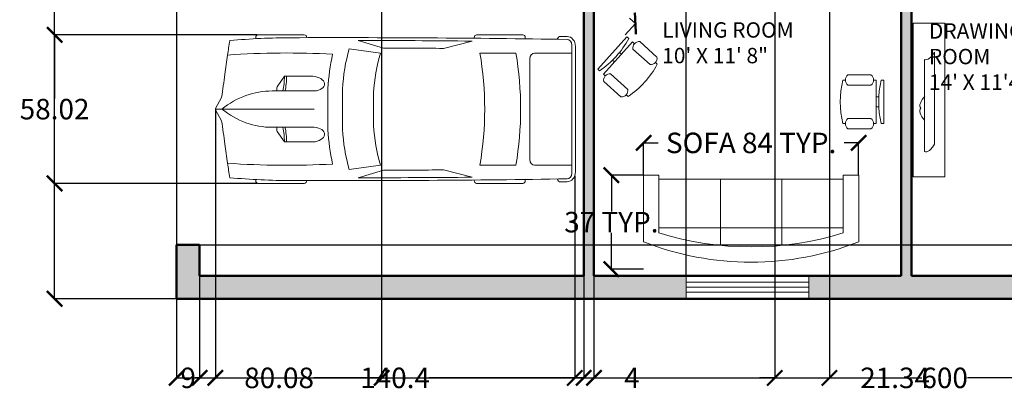
# Model space of a CAD drawing. Units: inches. Extents: x -30 to 744, y -375 to 57.
# Tile 1 of 8: x -30 to 355, y -375 to -230. Entities that reach past the tile are written whole.
import ezdxf

# ---------------------------------------------------------------- set-up
doc = ezdxf.new("R2010")
doc.units = ezdxf.units.IN
doc.header["$MEASUREMENT"] = 0
for name, color, linetype, lineweight in [('A-ANNO-DIMS', 2, 'Continuous', 18), ('A-AREA-IDEN', 7, 'Continuous', 25), ('A-EQPM-VEHI', 8, 'Continuous', 13), ('A-FURN', 8, 'Continuous', 18), ('A-GLAZ', 4, 'Continuous', 18), ('A-WALL', 7, 'Continuous', 50)]:
    doc.layers.add(name, color=color, linetype=linetype, lineweight=lineweight)
doc.layers.add('A-WALL-PATT', color=251, linetype='Continuous', lineweight=13, true_color=0x636466)
doc.styles.get("Standard").update_dxf_attribs({"font": 'arial.ttf'})
doc.dimstyles.get("Standard").update_dxf_attribs({"dimtxt": 8, "dimasz": 6, "dimexe": 0.18, "dimexo": 0.0625, "dimgap": 0.09, "dimtad": 0, "dimtih": 1, "dimtoh": 1, "dimdec": 0, "dimzin": 0, "dimdsep": 46, "dimlunit": 4, "dimtxsty": 'Standard', "dimblk": 'ARCHTICK', "dimcen": 0.09, "dimadec": 0, "dimazin": 0, "dimtfac": 1, "dimtdec": 0, "dimtofl": 0, "dimtmove": 0, "dimatfit": 1, "dimldrblk": 'ARCHTICK', "dimfxl": 1, "dimtolj": 1, "dimtzin": 0, "dimarcsym": 0})

# ---------------------------------------------------------------- blocks, each defined once
blk = doc.blocks.new('Sofa - Roundback 7 ft.')
for p, q in [((-12.00002, -32.4421), (-12.00003, -6.5971)), ((11.99997, -32.4421), (11.99998, -6.5971)), ((-36.000027, -34), (-36.000027, -11.4696)), ((35.99998, -34), (35.99998, -11.4696)), ((-35.999844, -13.3819), (35.9998, -13.3819)), ((-36.000027, -32.4421), (35.99998, -32.4421))]:
    blk.add_line(p, q)
for points in [[(-36.000027, -34), (-42.000027, -34), (-42.000027, -8)], [(41.99998, -8), (41.99998, -34), (35.99998, -34)]]:
    blk.add_lwpolyline(points)
for centre, radius, start, end in [((0, -114.25), 114.25, 68.43141, 111.5686), ((-0.00001, -127.1968), 121.1968, 72.72033, 107.2797)]:
    blk.add_arc(centre, radius, start, end)
blk = doc.blocks.new('Chair - Desk')
for p, q in [((-8.5, 0), (-8.5, -1)), ((-8.5, 0), (8.5, 0)), ((8.5, 0), (8.5, -1)), ((-8.5, -3), (-8.5, -4)), ((-8.5, -3), (8.5, -3)), ((-2, -3), (-2, -1.9355)), ((2, -1.9576), (2, -3)), ((8.5, -3), (8.5, -4)), ((-10.5, -5), (-10.5, -14)), ((-6.5, -14), (-6.5, -5)), ((6.5, -5), (6.5, -14)), ((10.5, -14), (10.5, -5)), ((-8.5, -15), (-8.5, -16)), ((8.5, -15), (8.5, -16))]:
    blk.add_line(p, q)
for centre, radius, start, end in [((0, 34.625), 36.625, 256.5803, 283.4197), ((-8.5, -6.5), 2.5, 36.8699, 143.1301), ((8.5, -6.5), 2.5, 36.8699, 143.1301), ((-8.5, -12.5), 2.5, 216.8699, 323.1301), ((8.5, -12.5), 2.5, 216.8699, 323.1301), ((0, 19.625), 36.625, 256.5803, 283.4197)]:
    blk.add_arc(centre, radius, start, end)
blk = doc.blocks.new('*U20')
for p, q in [((21.1, 37.41), (21.1, 36.83)), ((46.55, 38.89), (22.35, 38.89)), ((47.8, 37.39), (47.8, 37.41)), ((135.45, 37.07), (135.45, 37.41)), ((136.7, 38.89), (160.9, 38.89)), ((162.15, 37.41), (162.15, 36.77)), ((70.03, 31.54), (86.41, 29.35)), ((87.99, 31.87), (74.76, 35.92)), ((134.31, 35.6), (119.29, 31.78)), ((186.47, -33.5), (186.47, 33.5)), ((188.4, -32.76), (188.4, 32.76)), ((138.42, 29.35), (157.25, 29.35)), ((164.52, 26.39), (164.52, -26.39)), ((186.47, 29.35), (167.01, 29.35)), ((32.27, 11.63), (36.13, 17.17)), ((36.13, 17.17), (50.94, 17.17)), ((32.12, 9.51), (32.12, 11.15)), ((58.92, -10.77), (58.92, 10.77)), ((66.55, -10.53), (66.55, 10.53)), ((186.47, -10.53), (186.47, 10.53)), ((3.27, 6.13), (0.1, 0.41)), ((29.77, 9.51), (51.68, 9.51)), ((82.74, 8.5), (82.74, -8.5)), ((0, 0), (51.68, 0)), ((0.1, -0.41), (3.27, -6.13)), ((29.77, -9.51), (51.68, -9.51)), ((32.12, -9.51), (32.12, -11.15)), ((32.27, -11.63), (36.13, -17.17)), ((36.13, -17.17), (50.94, -17.17)), ((86.41, -29.35), (70.03, -31.54)), ((157.25, -29.35), (138.42, -29.35)), ((167.01, -29.35), (186.47, -29.35)), ((87.99, -31.87), (74.76, -35.92)), ((134.31, -35.6), (119.29, -31.78)), ((21.1, -37.41), (21.1, -36.83)), ((46.55, -38.89), (22.35, -38.89)), ((47.8, -37.39), (47.8, -37.41)), ((135.45, -37.07), (135.45, -37.41)), ((136.7, -38.89), (160.9, -38.89)), ((162.15, -37.41), (162.15, -36.77))]:
    blk.add_line(p, q)
for centre, major_axis, ratio, start_param, end_param in [((41.19, -490.86), (0, 528.23), 0.842304, 0.00281, 0.075598), ((22.35, 37.41), (0, -1.48), 0.842304, 3.141593, 4.712389), ((64.48, -10555.62), (0, 10593.03), 0.842304, -0.013397, 0.002797), ((46.55, 37.41), (0, 1.48), 0.842304, -1.570796, 0), ((136.7, 37.41), (0, -1.48), 0.842304, 3.141593, 4.712389), ((160.9, 37.41), (0, 1.48), 0.842304, -1.570796, 0), ((180.63, 35.84), (0, 2.22), 0.842304, -0.013017, 1.249894), ((64.48, -10556.36), (0, 10595.31), 0.842304, -0.013397, -0.013017), ((183.98, 33.5), (0, -2.96), 0.842304, 1.570796, 3.128196), ((183.98, 32.76), (0, -5.25), 0.842304, 1.570796, 3.128196), ((266.03, -27.52), (0, 313.31), 0.842304, 1.367076, 1.39176), ((135.29, 5.39), (0, 81.77), 0.842304, 1.245306, 1.50788), ((64.48, -10555.62), (0, -10591.55), 0.842304, 3.133765, 3.140441), ((95.79, -3666.35), (0, -3698.24), 0.842304, 3.134049, 3.144098), ((259.18, -27.52), (0, -305.3), 0.842304, 4.528606, 4.561838), ((37.47, -593.96), (0, -623.33), 0.842304, 3.096046, 3.200911), ((134.4, 5.39), (0, -89.78), 0.842304, 4.449482, 4.652344), ((149.6, 2.8), (0, -79.58), 0.842304, 4.372215, 4.640744), ((17.08, 0), (0, 147.02), 0.842304, 4.511394, 4.913384), ((35.91, 0), (0, 147.02), 0.842304, 4.511394, 4.913384), ((167.01, 26.39), (0, 2.96), 0.842304, 0, 1.570796), ((-204.49, 52.4), (0, -250.96), 0.842304, 1.385369, 1.434372), ((13.04, 17.01), (0, 27.42), 0.842304, 4.435146, 4.718221), ((14.2, 17.01), (0, 27.42), 0.842304, 4.435146, 4.718221), ((50.79, 13.34), (6.34, -0.36), 0.603834, -1.395552, 1.581315), ((32.75, 11.15), (0, 0.74), 0.842304, 0.879714, 1.570796), ((29.77, -46.66), (0, 56.17), 0.842304, 0, 0.590319), ((0.62, 0), (0, -0.74), 0.842304, 4.131459, 5.293319), ((29.77, 46.66), (0, 56.17), 0.842304, 2.551274, 3.141593), ((-204.49, -52.4), (0, 250.96), 0.842304, -1.434372, -1.385369), ((13.04, -17.01), (0, -27.42), 0.842304, 1.564964, 1.848039), ((14.2, -17.01), (0, -27.42), 0.842304, 1.564964, 1.848039), ((149.6, -2.8), (0, -79.58), 0.842304, -1.499151, -1.230623), ((32.75, -11.15), (0, -0.74), 0.842304, 4.712389, 5.403472), ((134.4, -5.39), (0, -89.78), 0.842304, -1.510751, -1.307889), ((135.29, -5.39), (0, -81.77), 0.842304, -1.50788, -1.245306), ((259.18, 27.52), (0, 305.3), 0.842304, 1.721348, 1.754579), ((266.03, 27.52), (0, 313.31), 0.842304, 1.749832, 1.774517), ((37.47, 593.96), (0, -623.33), 0.842304, -0.059319, 0.045547), ((167.01, -26.39), (0, -2.96), 0.842304, 4.712389, 6.283185), ((41.19, 490.86), (0, -528.23), 0.842304, -0.075598, -0.00281), ((64.48, 10555.62), (0, -10591.55), 0.842304, 0.001152, 0.007828), ((95.79, 3666.35), (0, -3698.24), 0.842304, -0.002505, 0.007544), ((183.98, -33.5), (0, 2.96), 0.842304, 3.15499, 4.712389), ((183.98, -32.76), (0, -5.25), 0.842304, 0.013397, 1.570796), ((22.35, -37.41), (0, 1.48), 0.842304, 1.570796, 3.141593), ((64.48, 10555.62), (0, 10593.03), 0.842304, 3.138796, 3.15499), ((46.55, -37.41), (0, -1.48), 0.842304, 0, 1.570796), ((136.7, -37.41), (0, -1.48), 0.842304, -1.570796, 0), ((160.9, -37.41), (0, 1.48), 0.842304, 3.141593, 4.712389), ((180.63, -35.84), (0, -2.22), 0.842304, -1.249894, 0.013017), ((64.48, 10556.36), (0, 10595.31), 0.842304, 3.15461, 3.15499)]:
    blk.add_ellipse(centre, major_axis=major_axis, ratio=ratio, start_param=start_param, end_param=end_param)
at = {"extrusion": (0, 0, -1)}
blk.add_ellipse((50.79, -13.34), major_axis=(6.34, 0.36), ratio=0.603834, start_param=-1.395552, end_param=1.581315, dxfattribs=at)
blk = doc.blocks.new('WIN-48IN')
for p, q in [((0, 0), (0, 48)), ((0, 48), (9, 48)), ((2.5, 48), (2.5, 0)), ((4.5, 48), (4.5, 0)), ((6.5, 48), (6.5, 0)), ((9, 48), (9, 0)), ((9, 48), (9, 0)), ((9, 0), (0, 0))]:
    blk.add_line(p, q)
blk = doc.blocks.new('TV-CONSOLE-60IN')
blk.add_lwpolyline([(0, 12.35), (60, 12.35), (60, 0), (0, 0)], close=True)
for points in [[(11.23, 8.37), (47.17, 8.37)], [(50.06, 4.48), (14.12, 4.48)]]:
    blk.add_lwpolyline(points)
for centre, major_axis in [((10.57, 6.42), (3.55, -1.95)), ((46.51, 6.42), (3.55, -1.95)), ((36.16, 5.7), (-3.02, -2.7))]:
    blk.add_ellipse(centre, major_axis=major_axis, ratio=0.501579, start_param=0, end_param=1.660459)
at = {"extrusion": (0, 0, -1)}
blk.add_ellipse((30.21, 5.79), major_axis=(2.93, -2.79), ratio=0.501579, start_param=0, end_param=1.660459, dxfattribs=at)
blk = doc.blocks.new('_ArchTick')
at = {"color": 0, "linetype": 'ByBlock', "const_width": 0.15}
blk.add_lwpolyline([(-0.5, -0.5), (0.5, 0.5)], dxfattribs=at)
blk = doc.blocks.new('*D28')
at = {"layer": 'A-ANNO-DIMS', "color": 0, "lineweight": -2, "transparency": 16777216}
for p, q in [((224.53, -216.2), (232.58, -207.3)), ((232.58, -207.3), (238.58, -207.3)), ((222.24, -214.13), (224.66, -216.32)), ((208.15, -229.7), (210.58, -231.89)), ((210.44, -231.77), (206.42, -236.22))]:
    blk.add_line(p, q, dxfattribs=at)
at = {"layer": 'Defpoints', "color": 0, "transparency": 16777216}
for p in [(222.2, -214.08), (224.53, -216.2), (208.11, -229.66)]:
    blk.add_point(p, dxfattribs=at)
at = {"layer": 'A-ANNO-DIMS', "color": 0, "lineweight": -2, "transparency": 16777216, "xscale": 6, "yscale": 6, "zscale": 6}
for p, rotation in [((224.53, -216.2), 227.8616521635315), ((210.44, -231.77), 47.86165216353145)]:
    blk.add_blockref('_ArchTick', p, dxfattribs=dict(at, rotation=rotation))
at = {"layer": 'A-ANNO-DIMS', "color": 0, "transparency": 16777216, "insert": (277.03, -207.3), "char_height": 8, "attachment_point": 5}
blk.add_mtext('\\A1;CHAIR 21 TYP.', dxfattribs=at)
blk = doc.blocks.new('*D34')
at = {"layer": 'A-ANNO-DIMS', "color": 0, "lineweight": -2, "transparency": 16777216}
for p, q in [((213.65, -290.99), (213.65, -278.27)), ((213.65, -278.45), (219.34, -278.45)), ((297.65, -278.45), (291.96, -278.45)), ((297.65, -290.99), (297.65, -278.27))]:
    blk.add_line(p, q, dxfattribs=at)
at = {"layer": 'Defpoints', "color": 0, "transparency": 16777216}
for p in [(213.65, -278.45), (213.65, -291.05), (297.65, -291.05)]:
    blk.add_point(p, dxfattribs=at)
at = {"layer": 'A-ANNO-DIMS', "color": 0, "lineweight": -2, "transparency": 16777216, "xscale": 6, "yscale": 6, "zscale": 6, "rotation": 180}
blk.add_blockref('_ArchTick', (213.65, -278.45), dxfattribs=at)
at = {"layer": 'A-ANNO-DIMS', "color": 0, "lineweight": -2, "transparency": 16777216, "xscale": 6, "yscale": 6, "zscale": 6}
blk.add_blockref('_ArchTick', (297.65, -278.45), dxfattribs=at)
at = {"layer": 'A-ANNO-DIMS', "color": 0, "transparency": 16777216, "insert": (255.65, -278.45), "char_height": 8, "attachment_point": 5}
blk.add_mtext('\\A1;SOFA 84 TYP.', dxfattribs=at)
blk = doc.blocks.new('*D35')
at = {"layer": 'A-ANNO-DIMS', "color": 0, "lineweight": -2, "transparency": 16777216}
for p, q in [((213.59, -291.05), (200.87, -291.05)), ((201.05, -291.05), (201.05, -305.21)), ((201.05, -327.72), (201.05, -313.56)), ((213.59, -327.72), (200.87, -327.72))]:
    blk.add_line(p, q, dxfattribs=at)
at = {"layer": 'Defpoints', "color": 0, "transparency": 16777216}
for p in [(213.65, -291.05), (201.05, -327.72), (213.65, -327.72)]:
    blk.add_point(p, dxfattribs=at)
at = {"layer": 'A-ANNO-DIMS', "color": 0, "lineweight": -2, "transparency": 16777216, "xscale": 6, "yscale": 6, "zscale": 6}
for p, rotation in [((201.05, -291.05), 90), ((201.05, -327.72), 270)]:
    blk.add_blockref('_ArchTick', p, dxfattribs=dict(at, rotation=rotation))
at = {"layer": 'A-ANNO-DIMS', "color": 0, "transparency": 16777216, "insert": (201.05, -309.38), "char_height": 8, "attachment_point": 5}
blk.add_mtext('\\A1;37 TYP.', dxfattribs=at)
blk = doc.blocks.new('*D60')
at = {"layer": 'A-ANNO-DIMS', "color": 0, "lineweight": -2, "transparency": 16777216}
for p, q in [((31.24, -339.36), (31.24, -370.38)), ((631.24, -339.36), (631.24, -370.38)), ((31.24, -370.2), (322.3, -370.2)), ((631.24, -370.2), (340.17, -370.2))]:
    blk.add_line(p, q, dxfattribs=at)
at = {"layer": 'Defpoints', "color": 0, "transparency": 16777216}
for p in [(31.24, -339.3), (631.24, -339.3), (631.24, -370.2)]:
    blk.add_point(p, dxfattribs=at)
at = {"layer": 'A-ANNO-DIMS', "color": 0, "lineweight": -2, "transparency": 16777216, "xscale": 6, "yscale": 6, "zscale": 6, "rotation": 180}
blk.add_blockref('_ArchTick', (31.24, -370.2), dxfattribs=at)
at = {"layer": 'A-ANNO-DIMS', "color": 0, "lineweight": -2, "transparency": 16777216, "xscale": 6, "yscale": 6, "zscale": 6}
blk.add_blockref('_ArchTick', (631.24, -370.2), dxfattribs=at)
at = {"layer": 'A-ANNO-DIMS', "color": 0, "transparency": 16777216, "insert": (331.24, -370.2), "char_height": 8, "attachment_point": 5}
blk.add_mtext('\\A1;600', dxfattribs=at)
blk = doc.blocks.new('*D61')
at = {"layer": 'A-ANNO-DIMS', "color": 0, "lineweight": -2, "transparency": 16777216}
for p, q in [((31.17, 20.7), (-16.61, 20.7)), ((-16.43, 20.7), (-16.43, -155.12)), ((-16.43, -339.3), (-16.43, -163.47)), ((31.17, -339.3), (-16.61, -339.3))]:
    blk.add_line(p, q, dxfattribs=at)
at = {"layer": 'Defpoints', "color": 0, "transparency": 16777216}
for p in [(-16.43, 20.7), (31.24, 20.7), (31.24, -339.3)]:
    blk.add_point(p, dxfattribs=at)
at = {"layer": 'A-ANNO-DIMS', "color": 0, "lineweight": -2, "transparency": 16777216, "xscale": 6, "yscale": 6, "zscale": 6}
for p, rotation in [((-16.43, 20.7), 90), ((-16.43, -339.3), 270)]:
    blk.add_blockref('_ArchTick', p, dxfattribs=dict(at, rotation=rotation))
at = {"layer": 'A-ANNO-DIMS', "color": 0, "transparency": 16777216, "insert": (-16.43, -159.3), "char_height": 8, "attachment_point": 5}
blk.add_mtext('\\A1;360', dxfattribs=at)
blk = doc.blocks.new('*D64')
at = {"layer": 'A-ANNO-DIMS', "color": 0, "lineweight": -2, "transparency": 16777216}
for p, q in [((40.3, -206.3), (662.32, -206.3)), ((662.14, -206.3), (662.14, -258.19)), ((662.14, -318.3), (662.14, -266.4)), ((40.3, -318.3), (662.32, -318.3))]:
    blk.add_line(p, q, dxfattribs=at)
at = {"layer": 'Defpoints', "color": 0, "transparency": 16777216}
for p in [(40.24, -206.3), (662.14, -206.3), (40.24, -318.3)]:
    blk.add_point(p, dxfattribs=at)
at = {"layer": 'A-ANNO-DIMS', "color": 0, "lineweight": -2, "transparency": 16777216, "xscale": 6, "yscale": 6, "zscale": 6}
for p, rotation in [((662.14, -206.3), 90), ((662.14, -318.3), 270)]:
    blk.add_blockref('_ArchTick', p, dxfattribs=dict(at, rotation=rotation))
at = {"layer": 'A-ANNO-DIMS', "color": 0, "transparency": 16777216, "insert": (662.14, -262.3), "char_height": 8, "attachment_point": 5}
blk.add_mtext('\\A1;112', dxfattribs=at)
blk = doc.blocks.new('*D65')
at = {"layer": 'A-ANNO-DIMS', "color": 0, "lineweight": -2, "transparency": 16777216}
for p, q in [((31.24, -132.36), (31.24, -370.38)), ((111.31, -143.36), (111.31, -370.38)), ((31.24, -370.2), (57.67, -370.2)), ((111.31, -370.2), (84.88, -370.2))]:
    blk.add_line(p, q, dxfattribs=at)
at = {"layer": 'Defpoints', "color": 0, "transparency": 16777216}
for p in [(31.24, -132.3), (111.31, -143.3), (111.31, -370.2)]:
    blk.add_point(p, dxfattribs=at)
at = {"layer": 'A-ANNO-DIMS', "color": 0, "lineweight": -2, "transparency": 16777216, "xscale": 6, "yscale": 6, "zscale": 6, "rotation": 180}
blk.add_blockref('_ArchTick', (31.24, -370.2), dxfattribs=at)
at = {"layer": 'A-ANNO-DIMS', "color": 0, "lineweight": -2, "transparency": 16777216, "xscale": 6, "yscale": 6, "zscale": 6}
blk.add_blockref('_ArchTick', (111.31, -370.2), dxfattribs=at)
at = {"layer": 'A-ANNO-DIMS', "color": 0, "transparency": 16777216, "insert": (71.27, -370.2), "char_height": 8, "attachment_point": 5}
blk.add_mtext('\\A1;80.08', dxfattribs=at)
blk = doc.blocks.new('*D67')
at = {"layer": 'A-ANNO-DIMS', "color": 0, "lineweight": -2, "transparency": 16777216}
for p, q in [((31.24, -318.36), (31.24, -370.38)), ((40.24, -318.36), (40.24, -370.38)), ((31.24, -370.2), (33.02, -370.2)), ((40.24, -370.2), (38.46, -370.2))]:
    blk.add_line(p, q, dxfattribs=at)
at = {"layer": 'Defpoints', "color": 0, "transparency": 16777216}
for p in [(31.24, -318.3), (40.24, -318.3), (40.24, -370.2)]:
    blk.add_point(p, dxfattribs=at)
at = {"layer": 'A-ANNO-DIMS', "color": 0, "lineweight": -2, "transparency": 16777216, "xscale": 6, "yscale": 6, "zscale": 6, "rotation": 180}
blk.add_blockref('_ArchTick', (31.24, -370.2), dxfattribs=at)
at = {"layer": 'A-ANNO-DIMS', "color": 0, "lineweight": -2, "transparency": 16777216, "xscale": 6, "yscale": 6, "zscale": 6}
blk.add_blockref('_ArchTick', (40.24, -370.2), dxfattribs=at)
at = {"layer": 'A-ANNO-DIMS', "color": 0, "transparency": 16777216, "insert": (35.74, -370.2), "char_height": 8, "attachment_point": 5}
blk.add_mtext('\\A1;9', dxfattribs=at)
blk = doc.blocks.new('*D68')
at = {"layer": 'A-ANNO-DIMS', "color": 0, "lineweight": -2, "transparency": 16777216}
for p, q in [((190.24, -330.36), (190.24, -370.38)), ((194.24, -330.36), (194.24, -370.38)), ((190.24, -370.2), (184.24, -370.2)), ((194.24, -370.2), (206.24, -370.2))]:
    blk.add_line(p, q, dxfattribs=at)
at = {"layer": 'Defpoints', "color": 0, "transparency": 16777216}
for p in [(190.24, -330.3), (194.24, -330.3), (194.24, -370.2)]:
    blk.add_point(p, dxfattribs=at)
at = {"layer": 'A-ANNO-DIMS', "color": 0, "lineweight": -2, "transparency": 16777216, "xscale": 6, "yscale": 6, "zscale": 6}
blk.add_blockref('_ArchTick', (190.24, -370.2), dxfattribs=at)
at = {"layer": 'A-ANNO-DIMS', "color": 0, "lineweight": -2, "transparency": 16777216, "xscale": 6, "yscale": 6, "zscale": 6, "rotation": 180}
blk.add_blockref('_ArchTick', (194.24, -370.2), dxfattribs=at)
at = {"layer": 'A-ANNO-DIMS', "color": 0, "transparency": 16777216, "insert": (209.09, -370.2), "char_height": 8, "attachment_point": 5}
blk.add_mtext('\\A1;4', dxfattribs=at)
blk = doc.blocks.new('*D73')
at = {"layer": 'A-ANNO-DIMS', "color": 0, "lineweight": -2, "transparency": 16777216}
for p, q in [((194.24, -330.23), (194.24, 51.78)), ((194.24, 51.6), (206.42, 51.6)), ((230.24, 51.6), (218.05, 51.6)), ((230.24, -330.23), (230.24, 51.78))]:
    blk.add_line(p, q, dxfattribs=at)
at = {"layer": 'Defpoints', "color": 0, "transparency": 16777216}
for p in [(230.24, 51.6), (194.24, -330.3), (230.24, -330.3)]:
    blk.add_point(p, dxfattribs=at)
at = {"layer": 'A-ANNO-DIMS', "color": 0, "lineweight": -2, "transparency": 16777216, "xscale": 6, "yscale": 6, "zscale": 6, "rotation": 180}
blk.add_blockref('_ArchTick', (194.24, 51.6), dxfattribs=at)
at = {"layer": 'A-ANNO-DIMS', "color": 0, "lineweight": -2, "transparency": 16777216, "xscale": 6, "yscale": 6, "zscale": 6}
blk.add_blockref('_ArchTick', (230.24, 51.6), dxfattribs=at)
at = {"layer": 'A-ANNO-DIMS', "color": 0, "transparency": 16777216, "insert": (212.24, 51.6), "char_height": 8, "attachment_point": 5}
blk.add_mtext('\\A1;36', dxfattribs=at)
blk = doc.blocks.new('*D74')
at = {"layer": 'A-ANNO-DIMS', "color": 0, "lineweight": -2, "transparency": 16777216}
for p, q in [((318.24, -330.23), (318.24, 51.78)), ((318.24, 51.6), (342.41, 51.6)), ((378.24, 51.6), (354.06, 51.6)), ((378.24, -330.23), (378.24, 51.78))]:
    blk.add_line(p, q, dxfattribs=at)
at = {"layer": 'Defpoints', "color": 0, "transparency": 16777216}
for p in [(378.24, 51.6), (318.24, -330.3), (378.24, -330.3)]:
    blk.add_point(p, dxfattribs=at)
at = {"layer": 'A-ANNO-DIMS', "color": 0, "lineweight": -2, "transparency": 16777216, "xscale": 6, "yscale": 6, "zscale": 6, "rotation": 180}
blk.add_blockref('_ArchTick', (318.24, 51.6), dxfattribs=at)
at = {"layer": 'A-ANNO-DIMS', "color": 0, "lineweight": -2, "transparency": 16777216, "xscale": 6, "yscale": 6, "zscale": 6}
blk.add_blockref('_ArchTick', (378.24, 51.6), dxfattribs=at)
at = {"layer": 'A-ANNO-DIMS', "color": 0, "transparency": 16777216, "insert": (348.24, 51.6), "char_height": 8, "attachment_point": 5}
blk.add_mtext('\\A1;60', dxfattribs=at)
blk = doc.blocks.new('*D87')
at = {"layer": 'A-ANNO-DIMS', "color": 0, "lineweight": -2, "transparency": 16777216}
for p, q in [((46.37, -265.33), (46.37, -370.38)), ((186.76, -291.29), (186.76, -370.38)), ((46.37, -370.2), (103.37, -370.2)), ((186.76, -370.2), (129.76, -370.2))]:
    blk.add_line(p, q, dxfattribs=at)
at = {"layer": 'Defpoints', "color": 0, "transparency": 16777216}
for p in [(46.37, -265.26), (186.76, -291.23), (186.76, -370.2)]:
    blk.add_point(p, dxfattribs=at)
at = {"layer": 'A-ANNO-DIMS', "color": 0, "lineweight": -2, "transparency": 16777216, "xscale": 6, "yscale": 6, "zscale": 6, "rotation": 180}
blk.add_blockref('_ArchTick', (46.37, -370.2), dxfattribs=at)
at = {"layer": 'A-ANNO-DIMS', "color": 0, "lineweight": -2, "transparency": 16777216, "xscale": 6, "yscale": 6, "zscale": 6}
blk.add_blockref('_ArchTick', (186.76, -370.2), dxfattribs=at)
at = {"layer": 'A-ANNO-DIMS', "color": 0, "transparency": 16777216, "insert": (116.57, -370.2), "char_height": 8, "attachment_point": 5}
blk.add_mtext('\\A1;140.4', dxfattribs=at)
blk = doc.blocks.new('*D88')
at = {"layer": 'A-ANNO-DIMS', "color": 0, "lineweight": -2, "transparency": 16777216}
for p, q in [((62.81, -236.25), (-16.61, -236.25)), ((-16.43, -236.25), (-16.43, -261.09)), ((-16.43, -294.27), (-16.43, -269.44)), ((62.81, -294.27), (-16.61, -294.27))]:
    blk.add_line(p, q, dxfattribs=at)
at = {"layer": 'Defpoints', "color": 0, "transparency": 16777216}
for p in [(62.87, -236.25), (-16.43, -294.27), (62.87, -294.27)]:
    blk.add_point(p, dxfattribs=at)
at = {"layer": 'A-ANNO-DIMS', "color": 0, "lineweight": -2, "transparency": 16777216, "xscale": 6, "yscale": 6, "zscale": 6}
for p, rotation in [((-16.43, -236.25), 90), ((-16.43, -294.27), 270)]:
    blk.add_blockref('_ArchTick', p, dxfattribs=dict(at, rotation=rotation))
at = {"layer": 'A-ANNO-DIMS', "color": 0, "transparency": 16777216, "insert": (-16.43, -265.26), "char_height": 8, "attachment_point": 5}
blk.add_mtext('\\A1;58.02', dxfattribs=at)
blk = doc.blocks.new('*D89')
at = {"layer": 'A-ANNO-DIMS', "color": 0, "lineweight": -2, "transparency": 16777216}
for p, q in [((264.9, -64.36), (264.9, -370.38)), ((286.24, -64.36), (286.24, -370.38)), ((264.9, -370.2), (258.9, -370.2)), ((286.24, -370.2), (298.24, -370.2))]:
    blk.add_line(p, q, dxfattribs=at)
at = {"layer": 'Defpoints', "color": 0, "transparency": 16777216}
for p in [(264.9, -64.3), (286.24, -64.3), (286.24, -370.2)]:
    blk.add_point(p, dxfattribs=at)
at = {"layer": 'A-ANNO-DIMS', "color": 0, "lineweight": -2, "transparency": 16777216, "xscale": 6, "yscale": 6, "zscale": 6}
blk.add_blockref('_ArchTick', (264.9, -370.2), dxfattribs=at)
at = {"layer": 'A-ANNO-DIMS', "color": 0, "lineweight": -2, "transparency": 16777216, "xscale": 6, "yscale": 6, "zscale": 6, "rotation": 180}
blk.add_blockref('_ArchTick', (286.24, -370.2), dxfattribs=at)
at = {"layer": 'A-ANNO-DIMS', "color": 0, "transparency": 16777216, "insert": (311.88, -370.2), "char_height": 8, "attachment_point": 5}
blk.add_mtext('\\A1;21.34', dxfattribs=at)

msp = doc.modelspace()

# ---------------------------------------------------------------- hatches: boundary and pattern name
at = {"layer": 'A-WALL-PATT'}
h = msp.add_hatch(color=256, dxfattribs=at)
h.dxf.hatch_style = 1
h.paths.add_polyline_path([(40.2356, 11.7031), (204.2356, 11.7031), (204.2356, -24.2969), (208.2356, -24.2969), (208.2356, 11.7031), (233.4275, 11.7031), (233.4275, 20.7031), (31.2356, 20.7031), (31.2356, -34.2969), (40.2356, -34.2969)])
h.paths.add_polyline_path([(40.2356, -82.2969), (31.2356, -82.2969), (31.2356, -132.2969), (40.2356, -132.2969), (51.0767, -132.2969), (111.3137, -132.2969), (111.3137, -143.2969), (120.3137, -143.2969), (120.3137, -132.2969), (156.2356, -132.2969), (156.2356, -128.2969), (113.6001, -128.2969), (113.6001, -128.3034), (53.6001, -128.3034), (40.2356, -128.2969)])
h.paths.add_polyline_path([(302.4681, 20.7031), (257.4275, 20.7031), (257.4275, 11.7031), (286.2356, 11.7031), (286.2356, -60.2969), (208.2356, -60.2969), (208.2356, -54.2969), (204.2356, -54.2969), (204.2356, -64.2969), (208.2356, -64.2969), (286.2356, -64.2969), (286.2356, -128.2969), (264.8954, -128.2969), (208.2356, -128.2969), (204.2356, -128.2969), (198.2356, -128.2969), (198.2356, -132.2969), (290.2356, -132.2969), (290.2356, -128.2969), (290.2356, 11.7031), (302.4681, 11.7031)])
h.paths.add_polyline_path([(405.515, 20.7031), (350.4681, 20.7031), (350.4681, 11.7031), (362.2356, 11.7031), (362.2356, -34.2969), (366.2356, -34.2969), (366.2356, 11.7031), (405.515, 11.7031)])
h.paths.add_polyline_path([(530.2713, 20.7031), (453.515, 20.7031), (453.515, 11.7031), (486.2356, 11.7031), (486.2356, -128.2969), (448.2356, -128.2969), (448.2356, -132.2969), (486.2356, -132.2969), (490.2356, -132.2969), (496.2356, -132.2969), (496.2356, -128.2969), (490.2356, -128.2969), (490.2356, 11.7031), (530.2713, 11.7031)])
h.paths.add_polyline_path([(631.2356, 20.7031), (578.2713, 20.7031), (578.2713, 11.7031), (622.2356, 11.7031), (622.2356, -37.4001), (631.2356, -37.4001)])
h.paths.add_polyline_path([(631.2356, -85.4001), (622.2356, -85.4001), (622.2356, -91.4001), (622.2356, -103.4001), (622.2356, -128.2969), (538.2356, -128.2969), (538.2356, -132.2969), (538.2356, -154.2969), (542.2356, -154.2969), (542.2356, -132.2969), (575.1375, -132.2969), (585.6313, -131.9348), (585.6438, -132.2969), (622.2356, -132.2969), (622.2356, -147.2969), (631.2356, -147.2969)])
h.paths.add_polyline_path([(631.2356, -171.2969), (622.2356, -171.2969), (622.2356, -185.4028), (622.2356, -186.2969), (622.2356, -190.2969), (542.2356, -190.2969), (542.2356, -184.2969), (538.2356, -184.2969), (538.2356, -190.2969), (538.2356, -194.2969), (622.2356, -194.2969), (622.2356, -237.4632), (631.2356, -237.4632)])
h.paths.add_polyline_path([(631.2356, -285.4632), (622.2356, -285.4632), (622.2356, -330.2969), (490.2356, -330.2969), (490.2356, -194.2969), (494.2356, -194.2969), (495.2356, -194.2969), (495.2356, -190.2969), (494.2356, -190.2969), (490.2356, -190.2969), (486.2356, -190.2969), (366.2356, -190.2969), (366.2356, -194.2969), (486.2356, -194.2969), (486.2356, -330.2969), (426.2356, -330.2969), (426.2356, -339.2969), (631.2356, -339.2969)])
h.paths.add_polyline_path([(378.2356, -330.2969), (318.2356, -330.2969), (318.2356, -194.2969), (324.2356, -194.2969), (324.2356, -190.2969), (318.2356, -190.2969), (314.2356, -190.2969), (314.2356, -194.2969), (314.2356, -330.2969), (278.2356, -330.2969), (278.2356, -339.2969), (378.2356, -339.2969)])
h.paths.add_polyline_path([(190.2356, -330.2969), (40.2356, -330.2969), (40.2356, -318.2969), (31.2356, -318.2969), (31.2356, -330.2969), (31.2356, -339.2969), (190.2356, -339.2969)])
h.paths.add_polyline_path([(230.2356, -330.2969), (194.2356, -330.2969), (194.2356, -194.2969), (194.2356, -190.2969), (190.2356, -190.2969), (184.2356, -190.2969), (184.2356, -194.2969), (190.2356, -194.2969), (190.2356, -339.2969), (230.2356, -339.2969)])
h.paths.add_polyline_path([(142.2356, -190.2969), (120.3137, -190.2969), (120.3137, -184.2969), (116.3137, -184.2969), (111.3137, -184.2969), (111.3137, -190.2969), (40.2356, -190.2969), (31.2356, -190.2969), (31.2356, -194.2969), (31.2356, -206.2969), (40.2356, -206.2969), (40.2356, -194.2969), (142.2356, -194.2969)])

# ---------------------------------------------------------------- linework, layer by layer
at = {"layer": 'A-WALL'}
for p, q in [((190.2356, -194.2969), (190.2356, -330.2969)), ((194.2356, -194.2969), (194.2356, -330.2969)), ((314.2356, -194.2969), (314.2356, -330.2969)), ((318.2356, -194.2969), (318.2356, -330.2969)), ((31.2356, -330.2969), (31.2356, -318.2969)), ((31.2356, -318.2969), (40.2356, -318.2969)), ((40.2356, -318.2969), (40.2356, -330.2969)), ((31.2356, -339.2969), (31.2356, -330.2969)), ((40.2356, -330.2969), (190.2356, -330.2969)), ((314.2356, -330.2969), (194.2356, -330.2969)), ((486.2356, -330.2969), (318.2356, -330.2969)), ((190.2356, -339.2969), (31.2356, -339.2969))]:
    msp.add_line(p, q, dxfattribs=at)
msp.add_lwpolyline([(31.2356, -132.2969), (31.2356, 20.7031), (631.2356, 20.7031), (631.2356, -339.2969), (190.2356, -339.2969)], dxfattribs=at)

# ---------------------------------------------------------------- block references
at = {"layer": 'A-EQPM-VEHI', "xscale": 0.7465390365388112, "yscale": 0.7465390365388112, "zscale": 0.7465390365388112}
msp.add_blockref('*U20', (46.3696, -265.2632), dxfattribs=at)
at = {"layer": 'A-FURN'}
for name, p, rotation in [('TV-CONSOLE-60IN', (318.9236, -231.7286), 269.9999999999999), ('Chair - Desk', (201.4256, -243.3203), 47.86165216353146), ('Chair - Desk', (307.4694, -262.415), 270), ('Sofa - Roundback 7 ft.', (255.6524, -325.0507), 180)]:
    msp.add_blockref(name, p, dxfattribs=dict(at, rotation=rotation))
at = {"layer": 'A-GLAZ', "rotation": 270}
msp.add_blockref('WIN-48IN', (230.2357, -330.2973), dxfattribs=at)

# ---------------------------------------------------------------- texts
at = {"layer": 'A-AREA-IDEN', "char_height": 6, "attachment_point": 1}
for s, width, insert in [('LIVING ROOM \\P10\' X 11\' 8"', 81.553956, (220.9155, -231.3479)), ('DRAWING ROOM \\P14\' X 11\'4"', 61.140655, (325.0959, -231.7288))]:
    msp.add_mtext_dynamic_manual_height_columns(s, width=width, gutter_width=1, heights=[0], dxfattribs=dict(at, insert=insert))

# ---------------------------------------------------------------- dimensions: what is measured, and where the dimension line sits
at = {"layer": 'A-ANNO-DIMS'}
for base, p1, p2, override, picture, middle in [((230.2356, 51.6031), (194.2356, -330.2969), (230.2356, -330.2969), {"dimdec": 0, "dimlfac": 1, "dimrnd": 0, "dimzin": 0, "dimdsep": 46, "dimlunit": 2}, '*D73', (212.2356, 51.6031)), ((378.2356, 51.6031), (318.2356, -330.2969), (378.2356, -330.2969), {"dimdec": 0, "dimlfac": 1, "dimrnd": 0, "dimzin": 0, "dimdsep": 46, "dimlunit": 2}, '*D74', (348.2356, 51.6031)), ((286.2356, -370.1969), (264.8954, -64.2969), (286.2356, -64.2969), {"dimdec": 2, "dimlfac": 1, "dimrnd": 0, "dimzin": 0, "dimdsep": 46, "dimlunit": 2}, '*D89', (311.8754, -370.1969)), ((111.3137, -370.1969), (31.2356, -132.2969), (111.3137, -143.2969), {"dimdec": 2, "dimlfac": 1, "dimrnd": 0, "dimzin": 0, "dimdsep": 46, "dimlunit": 2}, '*D65', (71.2746, -370.1969)), ((186.762, -370.1969), (46.3696, -265.2632), (186.762, -291.2306), {"dimdec": 1, "dimlfac": 1, "dimrnd": 0, "dimzin": 0, "dimdsep": 46, "dimlunit": 2}, '*D87', (116.5658, -370.1969)), ((40.2356, -370.1969), (31.2356, -318.2969), (40.2356, -318.2969), {"dimdec": 0, "dimlfac": 1, "dimrnd": 0, "dimzin": 0, "dimdsep": 46, "dimlunit": 2}, '*D67', (35.7356, -370.1969)), ((194.2356, -370.1969), (190.2356, -330.2969), (194.2356, -330.2969), {"dimdec": 0, "dimlfac": 1, "dimrnd": 0, "dimzin": 0, "dimdsep": 46, "dimlunit": 2}, '*D68', (209.0923, -370.1969)), ((631.2356, -370.1969), (31.2356, -339.2969), (631.2356, -339.2969), {"dimdec": 0, "dimlfac": 1, "dimrnd": 0, "dimzin": 0, "dimdsep": 46, "dimlunit": 2}, '*D60', (331.2356, -370.1969))]:
    dim = msp.add_linear_dim(base=base, p1=p1, p2=p2, dimstyle='Standard', override=override, dxfattribs=at)
    dim.commit()
    dim.dimension.update_dxf_attribs({"geometry": picture, "text_midpoint": middle})
for base, p1, p2, override, picture, middle in [((-16.4253, 20.7031), (31.2356, -339.2969), (31.2356, 20.7031), {"dimdec": 0, "dimlfac": 1, "dimrnd": 0, "dimzin": 0, "dimdsep": 46, "dimlunit": 2}, '*D61', (-16.4253, -159.2969)), ((662.1356, -206.2969), (40.2356, -318.2969), (40.2356, -206.2969), {"dimdec": 0, "dimlfac": 1, "dimrnd": 0, "dimzin": 0, "dimdsep": 46, "dimlunit": 2}, '*D64', (662.1356, -262.2969)), ((-16.4253, -294.2735), (62.8728, -236.2528), (62.8728, -294.2735), {"dimdec": 2, "dimlfac": 1, "dimrnd": 0, "dimzin": 0, "dimdsep": 46, "dimlunit": 2}, '*D88', (-16.4253, -265.2632))]:
    dim = msp.add_linear_dim(base=base, p1=p1, p2=p2, angle=90, dimstyle='Standard', override=override, dxfattribs=at)
    dim.commit()
    dim.dimension.update_dxf_attribs({"geometry": picture, "text_midpoint": middle})
for base, p1, p2, angle, text, picture, middle in [((224.5309, -216.1978), (208.1057, -229.6565), (222.1951, -214.0844), 47.861652, 'CHAIR <> TYP.', '*D28', (277.0349, -207.2995)), ((213.6524, -278.4507), (297.6524, -291.0507), (213.6524, -291.0507), 180, 'SOFA <> TYP.', '*D34', (255.6524, -278.4507)), ((201.0524, -327.7173), (213.6524, -291.0507), (213.6524, -327.7173), 270, '<> TYP.', '*D35', (201.0524, -309.384))]:
    dim = msp.add_linear_dim(base=base, p1=p1, p2=p2, angle=angle, text=text, dimstyle='Standard', override={"dimdec": 0, "dimlfac": 1, "dimrnd": 0, "dimzin": 0, "dimdsep": 46, "dimlunit": 2}, dxfattribs=at)
    dim.commit()
    dim.dimension.update_dxf_attribs({"geometry": picture, "text_midpoint": middle})

doc.saveas('drawing.dxf')
